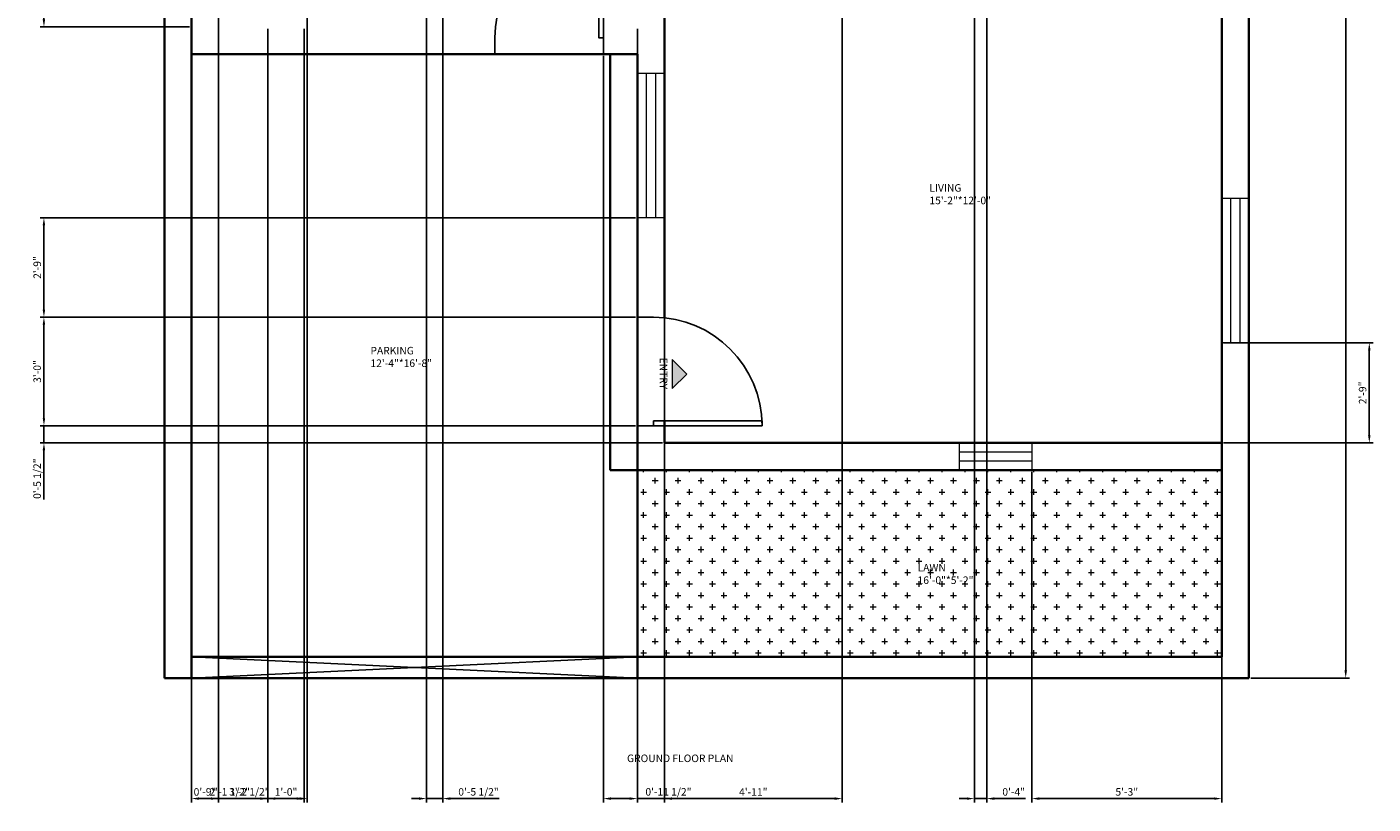
# Model space of a CAD drawing. Units: inches. Extents: x 2162 to 2610, y 1546 to 2356.
# Tile 1 of 3: x 2162 to 2609, y 1546 to 1804. Entities that reach past the tile are written whole.
import ezdxf

# ---------------------------------------------------------------- set-up
doc = ezdxf.new("R2010")
doc.units = ezdxf.units.IN
for name, color, linetype, lineweight in [('A-ANNO-DIMS', 2, 'Continuous', 18), ('A-ANNO-PATT', 7, 'Continuous', 13), ('A-ANNO-SYMB', 7, 'Continuous', 18), ('A-ANNO-TEXT', 7, 'Continuous', 25), ('A-AREA-IDEN', 7, 'Continuous', 18), ('A-DOOR', 3, 'Continuous', 25), ('A-GLAZ', 4, 'Continuous', 18), ('A-WALL', 7, 'Continuous', 35), ('L-PLNT-PATT', 9, 'Continuous', 13)]:
    doc.layers.add(name, color=color, linetype=linetype, lineweight=lineweight)
doc.styles.get("Standard").update_dxf_attribs({"font": 'arial.ttf'})
doc.dimstyles.new('ISO-25', dxfattribs={"dimtxt": 2.5, "dimasz": 2.5, "dimexe": 1.25, "dimexo": 0.625, "dimtad": 1, "dimdec": 1, "dimlunit": 3, "dimtxsty": 'Standard', "dimcen": 2.5, "dimadec": 0, "dimazin": 0, "dimtfac": 1, "dimtdec": 1, "dimtmove": 0, "dimatfit": 3, "dimfxl": 1, "dimarcsym": 0})

# ---------------------------------------------------------------- blocks, each defined once
blk = doc.blocks.new('*U2')
for p, q in [((0, 0), (0, -6)), ((40, 0), (40, -6))]:
    blk.add_line(p, q)
blk.add_lwpolyline([(0, 0), (0, 40), (1.75, 40), (1.75, 0)], close=True)
blk.add_arc((0, 0), 40, 0, 90)
blk = doc.blocks.new('*D5')
at = {"layer": 'A-ANNO-DIMS', "color": 0, "lineweight": -2, "transparency": 16777216}
for p, q in [((2568.49, 2308.05), (2601.29, 2308.05)), ((2600.04, 2305.55), (2600.04, 1590.55)), ((2568.49, 1588.05), (2601.29, 1588.05))]:
    blk.add_line(p, q, dxfattribs=at)
at = {"layer": 'A-ANNO-DIMS', "color": 0, "transparency": 16777216}
for points in [[(2599.62, 2305.55), (2600.45, 2305.55), (2600.04, 2308.05)], [(2599.62, 1590.55), (2600.45, 1590.55), (2600.04, 1588.05)]]:
    blk.add_solid(points, dxfattribs=at)
at = {"layer": 'Defpoints', "color": 0, "transparency": 16777216}
for p in [(2567.87, 2308.05), (2567.87, 1588.05), (2600.04, 1588.05)]:
    blk.add_point(p, dxfattribs=at)
at = {"layer": 'A-ANNO-DIMS', "color": 0, "transparency": 16777216, "insert": (2598.14, 1948.05), "char_height": 2.5, "attachment_point": 5, "rotation": 90}
blk.add_mtext("60'", dxfattribs=at)
blk = doc.blocks.new('WIN-48IN')
for p, q in [((0, 0), (0, 48)), ((0, 48), (9, 48)), ((3, 0), (3, 48)), ((6, 48), (6, 0)), ((9, 48), (9, 0)), ((9, 0), (0, 0))]:
    blk.add_line(p, q)
blk = doc.blocks.new('WIN-24IN')
for p, q in [((0, 9), (24, 9)), ((0, 0), (0, 9)), ((24, 9), (24, 0)), ((0, 6), (24, 6)), ((24, 3), (0, 3)), ((24, 0), (0, 0))]:
    blk.add_line(p, q)
blk = doc.blocks.new('*D24')
at = {"layer": 'A-ANNO-DIMS', "color": 0, "lineweight": -2, "transparency": 16777216}
for p, q in [((2364.24, 1707.75), (2166.62, 1707.75)), ((2167.87, 1674.25), (2167.87, 1705.25)), ((2364.24, 1671.75), (2166.62, 1671.75))]:
    blk.add_line(p, q, dxfattribs=at)
at = {"layer": 'A-ANNO-DIMS', "color": 0, "transparency": 16777216}
for points in [[(2167.45, 1705.25), (2168.28, 1705.25), (2167.87, 1707.75)], [(2167.45, 1674.25), (2168.28, 1674.25), (2167.87, 1671.75)]]:
    blk.add_solid(points, dxfattribs=at)
at = {"layer": 'Defpoints', "color": 0, "transparency": 16777216}
for p in [(2167.87, 1707.75), (2364.87, 1707.75), (2364.87, 1671.75)]:
    blk.add_point(p, dxfattribs=at)
at = {"layer": 'A-ANNO-DIMS', "color": 0, "transparency": 16777216, "insert": (2165.96, 1689.75), "char_height": 2.5, "attachment_point": 5, "rotation": 90}
blk.add_mtext('3\'-0"', dxfattribs=at)
blk = doc.blocks.new('*D26')
at = {"layer": 'A-ANNO-DIMS', "color": 0, "lineweight": -2, "transparency": 16777216}
for p, q in [((2432.87, 1896.22), (2432.87, 1546.8)), ((2373.87, 1890.43), (2373.87, 1546.8)), ((2376.37, 1548.05), (2430.37, 1548.05))]:
    blk.add_line(p, q, dxfattribs=at)
at = {"layer": 'A-ANNO-DIMS', "color": 0, "transparency": 16777216}
for points in [[(2376.37, 1548.47), (2376.37, 1547.63), (2373.87, 1548.05)], [(2430.37, 1548.47), (2430.37, 1547.63), (2432.87, 1548.05)]]:
    blk.add_solid(points, dxfattribs=at)
at = {"layer": 'Defpoints', "color": 0, "transparency": 16777216}
for p in [(2432.87, 1896.85), (2373.87, 1891.05), (2432.87, 1548.05)]:
    blk.add_point(p, dxfattribs=at)
at = {"layer": 'A-ANNO-DIMS', "color": 0, "transparency": 16777216, "insert": (2403.37, 1549.93), "char_height": 2.5, "attachment_point": 5}
blk.add_mtext('4\'-11"', dxfattribs=at)
blk = doc.blocks.new('*D29')
at = {"layer": 'A-ANNO-DIMS', "color": 0, "lineweight": -2, "transparency": 16777216}
for p, q in [((2216.24, 1823.87), (2166.62, 1823.87)), ((2167.87, 1821.37), (2167.87, 1806.55)), ((2216.24, 1804.05), (2166.62, 1804.05))]:
    blk.add_line(p, q, dxfattribs=at)
at = {"layer": 'A-ANNO-DIMS', "color": 0, "transparency": 16777216}
for points in [[(2167.45, 1821.37), (2168.28, 1821.37), (2167.87, 1823.87)], [(2167.45, 1806.55), (2168.28, 1806.55), (2167.87, 1804.05)]]:
    blk.add_solid(points, dxfattribs=at)
at = {"layer": 'Defpoints', "color": 0, "transparency": 16777216}
for p in [(2216.87, 1823.87), (2167.87, 1804.05), (2216.87, 1804.05)]:
    blk.add_point(p, dxfattribs=at)
at = {"layer": 'A-ANNO-DIMS', "color": 0, "transparency": 16777216, "insert": (2165.97, 1813.96), "char_height": 2.5, "attachment_point": 5, "rotation": 90}
blk.add_mtext('1\'-8"', dxfattribs=at)
blk = doc.blocks.new('*D33')
at = {"layer": 'A-ANNO-DIMS', "color": 0, "lineweight": -2, "transparency": 16777216}
for p, q in [((2559.49, 1699.24), (2609.12, 1699.24)), ((2607.87, 1696.74), (2607.87, 1668.55)), ((2559.49, 1666.05), (2609.12, 1666.05))]:
    blk.add_line(p, q, dxfattribs=at)
at = {"layer": 'A-ANNO-DIMS', "color": 0, "transparency": 16777216}
for points in [[(2607.45, 1696.74), (2608.28, 1696.74), (2607.87, 1699.24)], [(2607.45, 1668.55), (2608.28, 1668.55), (2607.87, 1666.05)]]:
    blk.add_solid(points, dxfattribs=at)
at = {"layer": 'Defpoints', "color": 0, "transparency": 16777216}
for p in [(2558.87, 1699.24), (2558.87, 1666.05), (2607.87, 1666.05)]:
    blk.add_point(p, dxfattribs=at)
at = {"layer": 'A-ANNO-DIMS', "color": 0, "transparency": 16777216, "insert": (2605.97, 1682.65), "char_height": 2.5, "attachment_point": 5, "rotation": 90}
blk.add_mtext('2\'-9"', dxfattribs=at)
blk = doc.blocks.new('*D34')
at = {"layer": 'A-ANNO-DIMS', "color": 0, "lineweight": -2, "transparency": 16777216}
for p, q in [((2364.24, 1740.74), (2166.62, 1740.74)), ((2167.87, 1738.24), (2167.87, 1710.25)), ((2364.24, 1707.75), (2166.62, 1707.75))]:
    blk.add_line(p, q, dxfattribs=at)
at = {"layer": 'A-ANNO-DIMS', "color": 0, "transparency": 16777216}
for points in [[(2167.45, 1738.24), (2168.28, 1738.24), (2167.87, 1740.74)], [(2167.45, 1710.25), (2168.28, 1710.25), (2167.87, 1707.75)]]:
    blk.add_solid(points, dxfattribs=at)
at = {"layer": 'Defpoints', "color": 0, "transparency": 16777216}
for p in [(2364.87, 1740.74), (2167.87, 1707.75), (2364.87, 1707.75)]:
    blk.add_point(p, dxfattribs=at)
at = {"layer": 'A-ANNO-DIMS', "color": 0, "transparency": 16777216, "insert": (2165.97, 1724.24), "char_height": 2.5, "attachment_point": 5, "rotation": 90}
blk.add_mtext('2\'-9"', dxfattribs=at)
blk = doc.blocks.new('*D37')
at = {"layer": 'A-ANNO-DIMS', "color": 0, "lineweight": -2, "transparency": 16777216}
for p, q in [((2495.83, 1656.43), (2495.83, 1546.8)), ((2558.87, 1656.43), (2558.87, 1546.8)), ((2498.33, 1548.05), (2556.37, 1548.05))]:
    blk.add_line(p, q, dxfattribs=at)
at = {"layer": 'A-ANNO-DIMS', "color": 0, "transparency": 16777216}
for points in [[(2498.33, 1548.47), (2498.33, 1547.63), (2495.83, 1548.05)], [(2556.37, 1548.47), (2556.37, 1547.63), (2558.87, 1548.05)]]:
    blk.add_solid(points, dxfattribs=at)
at = {"layer": 'Defpoints', "color": 0, "transparency": 16777216}
for p in [(2495.83, 1657.05), (2558.87, 1657.05), (2558.87, 1548.05)]:
    blk.add_point(p, dxfattribs=at)
at = {"layer": 'A-ANNO-DIMS', "color": 0, "transparency": 16777216, "insert": (2527.35, 1549.95), "char_height": 2.5, "attachment_point": 5}
blk.add_mtext('5\'-3"', dxfattribs=at)
blk = doc.blocks.new('*D38')
at = {"layer": 'A-ANNO-DIMS', "color": 0, "lineweight": -2, "transparency": 16777216}
for p, q in [((2242.23, 1803.43), (2242.23, 1546.8)), ((2254.23, 1803.43), (2254.23, 1546.8)), ((2244.73, 1548.05), (2251.73, 1548.05))]:
    blk.add_line(p, q, dxfattribs=at)
at = {"layer": 'A-ANNO-DIMS', "color": 0, "transparency": 16777216}
for points in [[(2244.73, 1548.47), (2244.73, 1547.63), (2242.23, 1548.05)], [(2251.73, 1548.47), (2251.73, 1547.63), (2254.23, 1548.05)]]:
    blk.add_solid(points, dxfattribs=at)
at = {"layer": 'Defpoints', "color": 0, "transparency": 16777216}
for p in [(2242.23, 1804.05), (2254.23, 1804.05), (2254.23, 1548.05)]:
    blk.add_point(p, dxfattribs=at)
at = {"layer": 'A-ANNO-DIMS', "color": 0, "transparency": 16777216, "insert": (2248.23, 1549.95), "char_height": 2.5, "attachment_point": 5}
blk.add_mtext('1\'-0"', dxfattribs=at)
blk = doc.blocks.new('*D39')
at = {"layer": 'A-ANNO-DIMS', "color": 0, "lineweight": -2, "transparency": 16777216}
for p, q in [((2216.87, 1803.43), (2216.87, 1546.8)), ((2242.23, 1803.43), (2242.23, 1546.8)), ((2219.37, 1548.05), (2239.73, 1548.05))]:
    blk.add_line(p, q, dxfattribs=at)
at = {"layer": 'A-ANNO-DIMS', "color": 0, "transparency": 16777216}
for points in [[(2219.37, 1548.47), (2219.37, 1547.63), (2216.87, 1548.05)], [(2239.73, 1548.47), (2239.73, 1547.63), (2242.23, 1548.05)]]:
    blk.add_solid(points, dxfattribs=at)
at = {"layer": 'Defpoints', "color": 0, "transparency": 16777216}
for p in [(2216.87, 1804.05), (2242.23, 1804.05), (2242.23, 1548.05)]:
    blk.add_point(p, dxfattribs=at)
at = {"layer": 'A-ANNO-DIMS', "color": 0, "transparency": 16777216, "insert": (2229.55, 1549.97), "char_height": 2.5, "attachment_point": 5}
blk.add_mtext('2\'-1 1/2"', dxfattribs=at)
blk = doc.blocks.new('*D40')
at = {"layer": 'A-ANNO-DIMS', "color": 0, "lineweight": -2, "transparency": 16777216}
for p, q in [((2216.87, 1890.43), (2216.87, 1546.8)), ((2255.27, 1890.43), (2255.27, 1546.8)), ((2219.37, 1548.05), (2252.77, 1548.05))]:
    blk.add_line(p, q, dxfattribs=at)
at = {"layer": 'A-ANNO-DIMS', "color": 0, "transparency": 16777216}
for points in [[(2219.37, 1548.47), (2219.37, 1547.63), (2216.87, 1548.05)], [(2252.77, 1548.47), (2252.77, 1547.63), (2255.27, 1548.05)]]:
    blk.add_solid(points, dxfattribs=at)
at = {"layer": 'Defpoints', "color": 0, "transparency": 16777216}
for p in [(2216.87, 1891.05), (2255.27, 1891.05), (2255.27, 1548.05)]:
    blk.add_point(p, dxfattribs=at)
at = {"layer": 'A-ANNO-DIMS', "color": 0, "transparency": 16777216, "insert": (2236.07, 1549.97), "char_height": 2.5, "attachment_point": 5}
blk.add_mtext('3\'-2 1/2"', dxfattribs=at)
blk = doc.blocks.new('*D48')
at = {"layer": 'A-ANNO-DIMS', "color": 0, "lineweight": -2, "transparency": 16777216}
for p, q in [((2225.8, 1936.5), (2225.8, 1546.8)), ((2216.87, 1933.89), (2216.87, 1546.8)), ((2223.3, 1548.05), (2219.37, 1548.05))]:
    blk.add_line(p, q, dxfattribs=at)
at = {"layer": 'A-ANNO-DIMS', "color": 0, "transparency": 16777216}
for points in [[(2219.37, 1548.47), (2219.37, 1547.63), (2216.87, 1548.05)], [(2223.3, 1548.47), (2223.3, 1547.63), (2225.8, 1548.05)]]:
    blk.add_solid(points, dxfattribs=at)
at = {"layer": 'Defpoints', "color": 0, "transparency": 16777216}
for p in [(2225.8, 1937.12), (2216.87, 1934.51), (2216.87, 1548.05)]:
    blk.add_point(p, dxfattribs=at)
at = {"layer": 'A-ANNO-DIMS', "color": 0, "transparency": 16777216, "insert": (2221.33, 1549.95), "char_height": 2.5, "attachment_point": 5}
blk.add_mtext('0\'-9"', dxfattribs=at)
blk = doc.blocks.new('*D49')
at = {"layer": 'A-ANNO-DIMS', "color": 0, "lineweight": -2, "transparency": 16777216}
for p, q in [((2364.87, 1803.43), (2364.87, 1546.8)), ((2353.61, 1794.43), (2353.61, 1546.8)), ((2356.11, 1548.05), (2362.37, 1548.05)), ((2364.87, 1548.05), (2383.03, 1548.05))]:
    blk.add_line(p, q, dxfattribs=at)
at = {"layer": 'A-ANNO-DIMS', "color": 0, "transparency": 16777216}
for points in [[(2356.11, 1548.47), (2356.11, 1547.63), (2353.61, 1548.05)], [(2362.37, 1548.47), (2362.37, 1547.63), (2364.87, 1548.05)]]:
    blk.add_solid(points, dxfattribs=at)
at = {"layer": 'Defpoints', "color": 0, "transparency": 16777216}
for p in [(2364.87, 1804.05), (2353.61, 1795.05), (2364.87, 1548.05)]:
    blk.add_point(p, dxfattribs=at)
at = {"layer": 'A-ANNO-DIMS', "color": 0, "transparency": 16777216, "insert": (2375.2, 1549.97), "char_height": 2.5, "attachment_point": 5}
blk.add_mtext('0\'-11 1/2"', dxfattribs=at)
blk = doc.blocks.new('*D56')
at = {"layer": 'A-ANNO-DIMS', "color": 0, "lineweight": -2, "transparency": 16777216}
for p, q in [((2294.87, 2214.43), (2294.87, 1546.8)), ((2300.28, 2208.43), (2300.28, 1546.8)), ((2292.37, 1548.05), (2289.87, 1548.05)), ((2294.87, 1548.05), (2300.28, 1548.05)), ((2302.78, 1548.05), (2319.01, 1548.05))]:
    blk.add_line(p, q, dxfattribs=at)
at = {"layer": 'A-ANNO-DIMS', "color": 0, "transparency": 16777216}
for points in [[(2292.37, 1548.47), (2292.37, 1547.63), (2294.87, 1548.05)], [(2302.78, 1548.47), (2302.78, 1547.63), (2300.28, 1548.05)]]:
    blk.add_solid(points, dxfattribs=at)
at = {"layer": 'Defpoints', "color": 0, "transparency": 16777216}
for p in [(2294.87, 2215.05), (2300.28, 2209.05), (2300.28, 1548.05)]:
    blk.add_point(p, dxfattribs=at)
at = {"layer": 'A-ANNO-DIMS', "color": 0, "transparency": 16777216, "insert": (2312.14, 1549.97), "char_height": 2.5, "attachment_point": 5}
blk.add_mtext('0\'-5 1/2"', dxfattribs=at)
blk = doc.blocks.new('*D57')
at = {"layer": 'A-ANNO-DIMS', "color": 0, "lineweight": -2, "transparency": 16777216}
for p, q in [((2480.87, 2214.43), (2480.87, 1546.8)), ((2476.76, 2208.43), (2476.76, 1546.8)), ((2474.26, 1548.05), (2471.76, 1548.05)), ((2476.76, 1548.05), (2480.87, 1548.05)), ((2483.37, 1548.05), (2493.76, 1548.05))]:
    blk.add_line(p, q, dxfattribs=at)
at = {"layer": 'A-ANNO-DIMS', "color": 0, "transparency": 16777216}
for points in [[(2474.26, 1548.47), (2474.26, 1547.63), (2476.76, 1548.05)], [(2483.37, 1548.47), (2483.37, 1547.63), (2480.87, 1548.05)]]:
    blk.add_solid(points, dxfattribs=at)
at = {"layer": 'Defpoints', "color": 0, "transparency": 16777216}
for p in [(2480.87, 2215.05), (2476.76, 2209.05), (2480.87, 1548.05)]:
    blk.add_point(p, dxfattribs=at)
at = {"layer": 'A-ANNO-DIMS', "color": 0, "transparency": 16777216, "insert": (2489.81, 1549.95), "char_height": 2.5, "attachment_point": 5}
blk.add_mtext('0\'-4"', dxfattribs=at)
blk = doc.blocks.new('*D61')
at = {"layer": 'A-ANNO-DIMS', "color": 0, "lineweight": -2, "transparency": 16777216}
for p, q in [((2167.87, 1674.25), (2167.87, 1676.75)), ((2364.24, 1671.75), (2166.62, 1671.75)), ((2167.87, 1671.75), (2167.87, 1666.05)), ((2373.24, 1666.05), (2166.62, 1666.05)), ((2167.87, 1663.55), (2167.87, 1647.33))]:
    blk.add_line(p, q, dxfattribs=at)
at = {"layer": 'A-ANNO-DIMS', "color": 0, "transparency": 16777216}
for points in [[(2167.45, 1674.25), (2168.28, 1674.25), (2167.87, 1671.75)], [(2167.45, 1663.55), (2168.28, 1663.55), (2167.87, 1666.05)]]:
    blk.add_solid(points, dxfattribs=at)
at = {"layer": 'Defpoints', "color": 0, "transparency": 16777216}
for p in [(2364.87, 1671.75), (2167.87, 1666.05), (2373.87, 1666.05)]:
    blk.add_point(p, dxfattribs=at)
at = {"layer": 'A-ANNO-DIMS', "color": 0, "transparency": 16777216, "insert": (2165.95, 1654.19), "char_height": 2.5, "attachment_point": 5, "rotation": 90}
blk.add_mtext('0\'-5 1/2"', dxfattribs=at)

msp = doc.modelspace()

# ---------------------------------------------------------------- hatches: boundary and pattern name
at = {"layer": 'A-ANNO-PATT'}
h = msp.add_hatch(color=256, dxfattribs=at)
h.dxf.hatch_style = 1
h.paths.add_polyline_path([(2376.38, 1693.68), (2376.38, 1684.12), (2381.34, 1688.9)])
at = {"layer": 'L-PLNT-PATT'}
h = msp.add_hatch(dxfattribs=at)
h.set_pattern_fill('CROSS', color=256, scale=0.6)
h.paths.add_polyline_path([(2558.87, 1657.05), (2364.87, 1657.05), (2364.87, 1595.05), (2558.87, 1595.05)])
h.paths.add_polyline_path([(2456.9, 1617.88), (2475.36, 1617.88), (2475.36, 1627.21), (2456.9, 1627.21)], flags=24)

# ---------------------------------------------------------------- linework, layer by layer
at = {"layer": 'A-ANNO-SYMB'}
for p, q in [((2376.38, 1693.68), (2376.38, 1684.12)), ((2376.38, 1693.68), (2381.34, 1688.9)), ((2381.34, 1688.9), (2376.38, 1684.12))]:
    msp.add_line(p, q, dxfattribs=at)
at = {"layer": 'A-DOOR'}
for p, q in [((2216.87, 1595.05), (2364.87, 1588.05)), ((2216.87, 1588.05), (2364.87, 1595.05))]:
    msp.add_line(p, q, dxfattribs=at)
at = {"layer": 'A-WALL'}
for p, q in [((2207.87, 1588.05), (2207.87, 2308.05)), ((2567.87, 2308.05), (2567.87, 1588.05)), ((2216.87, 1588.05), (2216.87, 2299.05)), ((2558.87, 2299.05), (2558.87, 1595.05)), ((2373.87, 1707.57), (2373.87, 1891.05)), ((2364.87, 1795.05), (2216.87, 1795.05)), ((2355.87, 1657.05), (2355.87, 1795.05)), ((2364.87, 1588.05), (2364.87, 1795.05)), ((2373.87, 1666.05), (2373.87, 1673.32)), ((2558.87, 1666.05), (2373.87, 1666.05)), ((2558.87, 1657.05), (2355.87, 1657.05)), ((2558.87, 1595.05), (2216.87, 1595.05)), ((2567.87, 1588.05), (2207.87, 1588.05))]:
    msp.add_line(p, q, dxfattribs=at)

# ---------------------------------------------------------------- block references
at = {"layer": 'A-DOOR', "xscale": -0.9, "yscale": 0.9, "zscale": 0.9}
msp.add_blockref('*U2', (2353.61, 1800.45), dxfattribs=at)
at = {"layer": 'A-DOOR', "xscale": -0.9, "yscale": 0.9, "zscale": 0.9, "rotation": 270}
msp.add_blockref('*U2', (2370.27, 1671.75), dxfattribs=at)
at = {"layer": 'A-GLAZ'}
for name, p in [('WIN-48IN', (2364.87, 1740.74)), ('WIN-48IN', (2558.87, 1699.24)), ('WIN-24IN', (2471.83, 1657.05))]:
    msp.add_blockref(name, p, dxfattribs=at)

# ---------------------------------------------------------------- texts
at = {"layer": 'A-ANNO-TEXT', "insert": (2374.83, 1694.37), "char_height": 2.5, "attachment_point": 1, "rotation": 270}
msp.add_mtext_dynamic_manual_height_columns('ENTRY', width=24.2429, gutter_width=12.5, heights=[0], dxfattribs=at)
at = {"layer": 'A-ANNO-TEXT', "insert": (2361.44, 1562.66), "char_height": 2.5, "attachment_point": 1}
msp.add_mtext_dynamic_manual_height_columns('GROUND FLOOR PLAN', width=241.1616, gutter_width=12.5, heights=[0], dxfattribs=at)
at = {"layer": 'A-AREA-IDEN', "char_height": 2.5, "attachment_point": 1}
for s, width, insert in [('LIVING\\P15\'-2"*12\'-0"', 89.2953, (2461.83, 1751.9)), ('PARKING\\P12\'-4"*16\'-8"', 90.5791, (2276.27, 1697.91)), ('LAWN\\P16\'-0"*5\'-2"', 93.3788, (2457.9, 1625.92))]:
    msp.add_mtext_dynamic_manual_height_columns(s, width=width, gutter_width=12.5, heights=[0], dxfattribs=dict(at, insert=insert))

# ---------------------------------------------------------------- dimensions: what is measured, and where the dimension line sits
at = {"layer": 'A-ANNO-DIMS'}
for base, p1, p2, override, picture, middle in [((2600.04, 1588.05), (2567.87, 2308.05), (2567.87, 1588.05), {"dimclrd": 0, "dimclre": 0, "dimclrt": 0}, '*D5', (2598.14, 1948.05)), ((2167.87, 1804.05), (2216.87, 1823.87), (2216.87, 1804.05), {"dimdec": 1, "dimlfac": 1, "dimrnd": 0, "dimzin": 1, "dimdsep": 46, "dimlunit": 4, "dimfrac": 2}, '*D29', (2165.97, 1813.96)), ((2167.87, 1707.75), (2364.87, 1740.74), (2364.87, 1707.75), {"dimdec": 1, "dimlfac": 1, "dimrnd": 0, "dimzin": 1, "dimdsep": 46, "dimlunit": 4, "dimfrac": 2}, '*D34', (2165.97, 1724.24)), ((2167.87, 1707.75), (2364.87, 1671.75), (2364.87, 1707.75), {"dimdec": 1, "dimlfac": 1, "dimrnd": 0, "dimzin": 1, "dimdsep": 46, "dimlunit": 4, "dimfrac": 2}, '*D24', (2165.96, 1689.75)), ((2607.87, 1666.05), (2558.87, 1699.24), (2558.87, 1666.05), {"dimdec": 1, "dimlfac": 1, "dimrnd": 0, "dimzin": 1, "dimdsep": 46, "dimlunit": 4, "dimfrac": 2}, '*D33', (2605.97, 1682.65)), ((2167.87, 1666.05), (2364.87, 1671.75), (2373.87, 1666.05), {"dimdec": 1, "dimlfac": 1, "dimrnd": 0, "dimzin": 1, "dimdsep": 46, "dimlunit": 4, "dimfrac": 2}, '*D61', (2165.95, 1654.19))]:
    dim = msp.add_linear_dim(base=base, p1=p1, p2=p2, angle=90, dimstyle='ISO-25', override=override, dxfattribs=at)
    dim.commit()
    dim.dimension.update_dxf_attribs({"geometry": picture, "text_midpoint": middle})
for base, p1, p2, picture, middle in [((2300.28, 1548.05), (2294.87, 2215.05), (2300.28, 2209.05), '*D56', (2312.14, 1549.97)), ((2480.87, 1548.05), (2476.76, 2209.05), (2480.87, 2215.05), '*D57', (2489.81, 1549.95)), ((2216.87, 1548.05), (2225.8, 1937.12), (2216.87, 1934.51), '*D48', (2221.33, 1549.95)), ((2432.87, 1548.05), (2373.87, 1891.05), (2432.87, 1896.85), '*D26', (2403.37, 1549.93)), ((2255.27, 1548.05), (2216.87, 1891.05), (2255.27, 1891.05), '*D40', (2236.07, 1549.97)), ((2242.23, 1548.05), (2216.87, 1804.05), (2242.23, 1804.05), '*D39', (2229.55, 1549.97)), ((2254.23, 1548.05), (2242.23, 1804.05), (2254.23, 1804.05), '*D38', (2248.23, 1549.95)), ((2364.87, 1548.05), (2353.61, 1795.05), (2364.87, 1804.05), '*D49', (2375.2, 1549.97)), ((2558.87, 1548.05), (2495.83, 1657.05), (2558.87, 1657.05), '*D37', (2527.35, 1549.95))]:
    dim = msp.add_linear_dim(base=base, p1=p1, p2=p2, dimstyle='ISO-25', override={"dimdec": 1, "dimlfac": 1, "dimrnd": 0, "dimzin": 1, "dimdsep": 46, "dimlunit": 4, "dimfrac": 2}, dxfattribs=at)
    dim.commit()
    dim.dimension.update_dxf_attribs({"geometry": picture, "text_midpoint": middle})

doc.saveas('drawing.dxf')
